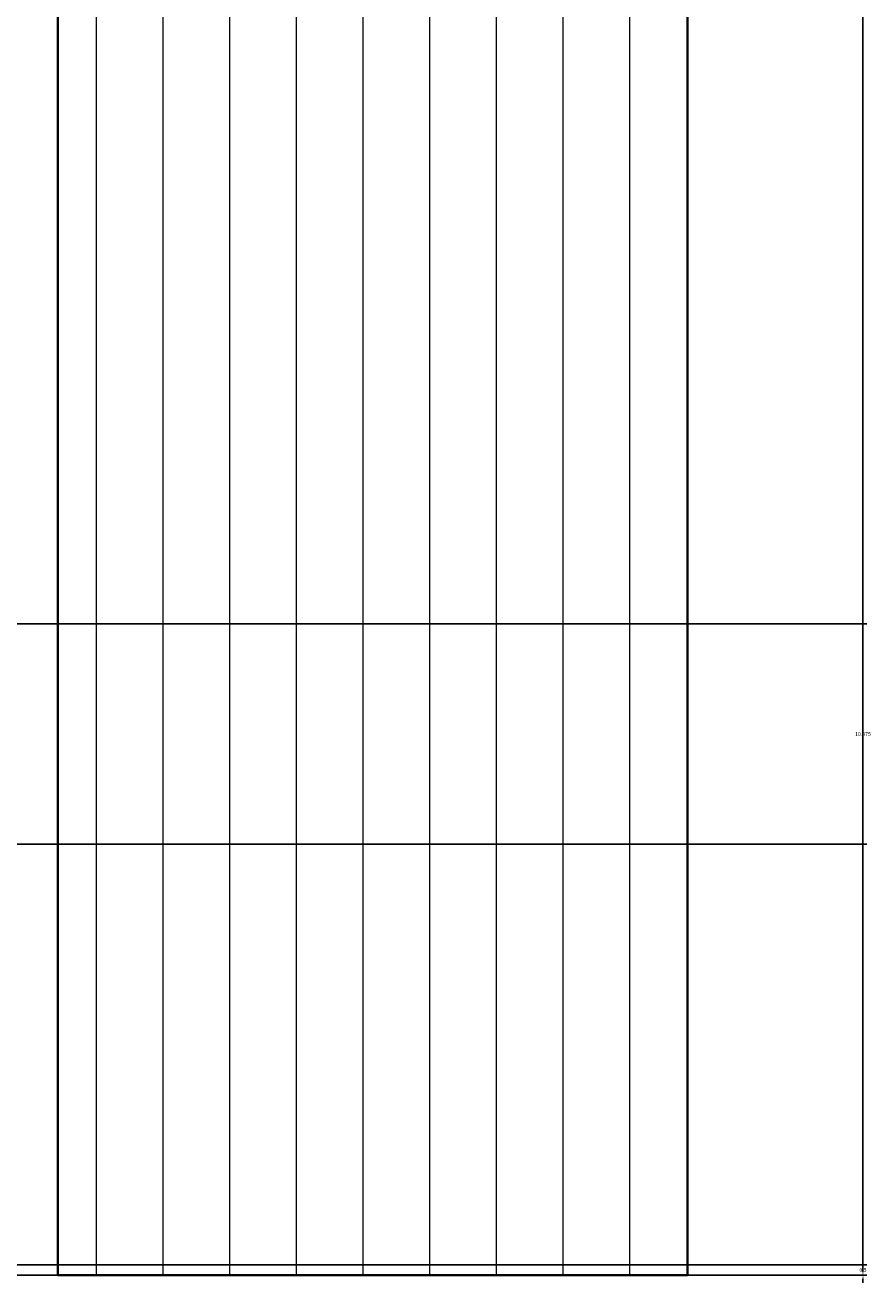
# Model space of a CAD drawing. Units: millimetres. Extents: x 446512 to 447461, y 70395 to 70610.
# Tile 9 of 39: x 446748 to 446788, y 70413 to 70473. Entities that reach past the tile are written whole.
import ezdxf

# ---------------------------------------------------------------- set-up
doc = ezdxf.new("R2010")
doc.units = ezdxf.units.MM
for name, color, linetype, lineweight in [('A-ANNO-DIMS', 2, 'Continuous', 18), ('A-FURN', 7, 'Continuous', 35), ('A-FURN-PATT', 38, 'Continuous', 13)]:
    doc.layers.add(name, color=color, linetype=linetype, lineweight=lineweight)
doc.styles.get("Standard").update_dxf_attribs({"font": 'arial.ttf'})
doc.dimstyles.get("Standard").update_dxf_attribs({"dimtxt": 0.18, "dimasz": 0.18, "dimexe": 0.18, "dimexo": 0.0625, "dimgap": 0.09, "dimtad": 0, "dimtih": 1, "dimtoh": 1, "dimdec": 4, "dimzin": 0, "dimdsep": 46, "dimtxsty": 'Standard', "dimcen": 0.09, "dimadec": 0, "dimazin": 0, "dimtfac": 1, "dimtdec": 4, "dimtofl": 0, "dimtmove": 0, "dimatfit": 3, "dimfxl": 1, "dimtolj": 1, "dimtzin": 0, "dimarcsym": 0})

# ---------------------------------------------------------------- blocks, each defined once
blk = doc.blocks.new('*D17')
at = {"layer": 'A-ANNO-DIMS', "color": 0, "lineweight": -2, "transparency": 16777216}
for p, q in [((446779.286, 70569.645), (446787.753, 70569.645)), ((446787.573, 70569.465), (446787.573, 70491.695)), ((446787.573, 70413.562), (446787.573, 70491.331)), ((446779.286, 70413.382), (446787.753, 70413.382))]:
    blk.add_line(p, q, dxfattribs=at)
at = {"layer": 'A-ANNO-DIMS', "color": 0, "transparency": 16777216}
for points in [[(446787.543, 70569.465), (446787.603, 70569.465), (446787.573, 70569.645)], [(446787.543, 70413.562), (446787.603, 70413.562), (446787.573, 70413.382)]]:
    blk.add_solid(points, dxfattribs=at)
at = {"layer": 'Defpoints', "color": 0, "transparency": 16777216}
for p in [(446779.223, 70569.645), (446787.573, 70569.645), (446779.223, 70413.382)]:
    blk.add_point(p, dxfattribs=at)
at = {"layer": 'A-ANNO-DIMS', "color": 0, "transparency": 16777216, "insert": (446787.573, 70491.513), "char_height": 0.18, "attachment_point": 5}
blk.add_mtext('\\A1;156.26', dxfattribs=at)
blk = doc.blocks.new('*D18')
at = {"layer": 'A-ANNO-DIMS', "color": 0, "lineweight": -2, "transparency": 16777216}
for p, q in [((446686.51, 70433.382), (446678.043, 70433.382)), ((446678.223, 70433.202), (446678.223, 70423.563)), ((446678.223, 70413.562), (446678.223, 70423.2)), ((446749.161, 70413.382), (446678.043, 70413.382))]:
    blk.add_line(p, q, dxfattribs=at)
at = {"layer": 'A-ANNO-DIMS', "color": 0, "transparency": 16777216}
for points in [[(446678.193, 70433.202), (446678.253, 70433.202), (446678.223, 70433.382)], [(446678.193, 70413.562), (446678.253, 70413.562), (446678.223, 70413.382)]]:
    blk.add_solid(points, dxfattribs=at)
at = {"layer": 'Defpoints', "color": 0, "transparency": 16777216}
for p in [(446678.223, 70433.382), (446686.573, 70433.382), (446749.223, 70413.382)]:
    blk.add_point(p, dxfattribs=at)
at = {"layer": 'A-ANNO-DIMS', "color": 0, "transparency": 16777216, "insert": (446678.223, 70423.382), "char_height": 0.18, "attachment_point": 5}
blk.add_mtext('\\A1;20', dxfattribs=at)
blk = doc.blocks.new('*D26')
at = {"layer": 'A-ANNO-DIMS', "color": 0, "lineweight": -2, "transparency": 16777216}
for p, q in [((446744.1, 70444.38), (446787.753, 70444.38)), ((446787.573, 70444.2), (446787.573, 70439.324)), ((446787.573, 70434.085), (446787.573, 70438.96)), ((446744.1, 70433.905), (446787.753, 70433.905))]:
    blk.add_line(p, q, dxfattribs=at)
at = {"layer": 'A-ANNO-DIMS', "color": 0, "transparency": 16777216}
for points in [[(446787.543, 70444.2), (446787.603, 70444.2), (446787.573, 70444.38)], [(446787.543, 70434.085), (446787.603, 70434.085), (446787.573, 70433.905)]]:
    blk.add_solid(points, dxfattribs=at)
at = {"layer": 'Defpoints', "color": 0, "transparency": 16777216}
for p in [(446744.038, 70444.38), (446787.573, 70444.38), (446744.038, 70433.905)]:
    blk.add_point(p, dxfattribs=at)
at = {"layer": 'A-ANNO-DIMS', "color": 0, "transparency": 16777216, "insert": (446787.573, 70439.142), "char_height": 0.18, "attachment_point": 5}
blk.add_mtext('\\A1;10.475', dxfattribs=at)
blk = doc.blocks.new('*D45')
at = {"layer": 'A-ANNO-DIMS', "color": 0, "lineweight": -2, "transparency": 16777216}
for p, q in [((446787.57348, 70414.06155), (446787.57348, 70414.24155)), ((446699.491325, 70413.38155), (446787.75348, 70413.38155)), ((446699.991325, 70413.88155), (446787.75348, 70413.88155)), ((446787.57348, 70413.20155), (446787.57348, 70413.02155))]:
    blk.add_line(p, q, dxfattribs=at)
at = {"layer": 'A-ANNO-DIMS', "color": 0, "transparency": 16777216}
for points in [[(446787.54348, 70414.06155), (446787.60348, 70414.06155), (446787.57348, 70413.88155)], [(446787.54348, 70413.20155), (446787.60348, 70413.20155), (446787.57348, 70413.38155)]]:
    blk.add_solid(points, dxfattribs=at)
at = {"layer": 'Defpoints', "color": 0, "transparency": 16777216}
for p in [(446699.428825, 70413.38155), (446699.928825, 70413.88155), (446787.57348, 70413.38155)]:
    blk.add_point(p, dxfattribs=at)
at = {"layer": 'A-ANNO-DIMS', "color": 0, "transparency": 16777216, "insert": (446787.57348, 70413.63155), "char_height": 0.18, "attachment_point": 5}
blk.add_mtext('\\A1;0.5', dxfattribs=at)

msp = doc.modelspace()

# ---------------------------------------------------------------- hatches: boundary and pattern name
at = {"layer": 'A-FURN-PATT'}
h = msp.add_hatch(dxfattribs=at)
h.set_pattern_fill('ANSI31', color=256, angle=45)
h.paths.add_polyline_path([(446779.2235, 70569.6449), (446749.2235, 70569.6449), (446749.2235, 70413.3815), (446779.2235, 70413.3815)])

# ---------------------------------------------------------------- linework, layer by layer
at = {"layer": 'A-FURN'}
for p, q in [((446749.2235, 70569.6449), (446749.2235, 70413.3815)), ((446779.2235, 70413.3815), (446779.2235, 70569.6449)), ((446749.2235, 70413.3815), (446753.8802, 70413.3815)), ((446749.2235, 70413.3815), (446779.2235, 70413.3815))]:
    msp.add_line(p, q, dxfattribs=at)

# ---------------------------------------------------------------- dimensions: what is measured, and where the dimension line sits
at = {"layer": 'A-ANNO-DIMS'}
for base, p1, p2, override, picture, middle in [((446787.5735, 70569.6449), (446779.2235, 70413.3815), (446779.2235, 70569.6449), {"dimdec": 2, "dimlfac": 1, "dimrnd": 0, "dimzin": 0, "dimdsep": 46, "dimlunit": 2}, '*D17', (446787.5735, 70491.5132)), ((446787.5735, 70444.3797), (446744.0375, 70433.9045), (446744.0375, 70444.3797), {"dimdec": 3, "dimlfac": 1, "dimrnd": 0, "dimzin": 0, "dimdsep": 46, "dimlunit": 2}, '*D26', (446787.5735, 70439.1421)), ((446678.2228, 70433.3816), (446749.2235, 70413.3815), (446686.5728, 70433.3816), {"dimdec": 0, "dimlfac": 1, "dimrnd": 0, "dimzin": 0, "dimdsep": 46, "dimlunit": 2}, '*D18', (446678.2228, 70423.3815)), ((446787.5735, 70413.3815), (446699.9288, 70413.8816), (446699.4288, 70413.3815), {"dimdec": 1, "dimlfac": 1, "dimrnd": 0, "dimzin": 0, "dimdsep": 46, "dimlunit": 2}, '*D45', (446787.5735, 70413.6315))]:
    dim = msp.add_linear_dim(base=base, p1=p1, p2=p2, angle=90, dimstyle='Standard', override=override, dxfattribs=at)
    dim.commit()
    dim.dimension.update_dxf_attribs({"geometry": picture, "text_midpoint": middle})

doc.saveas('drawing.dxf')
